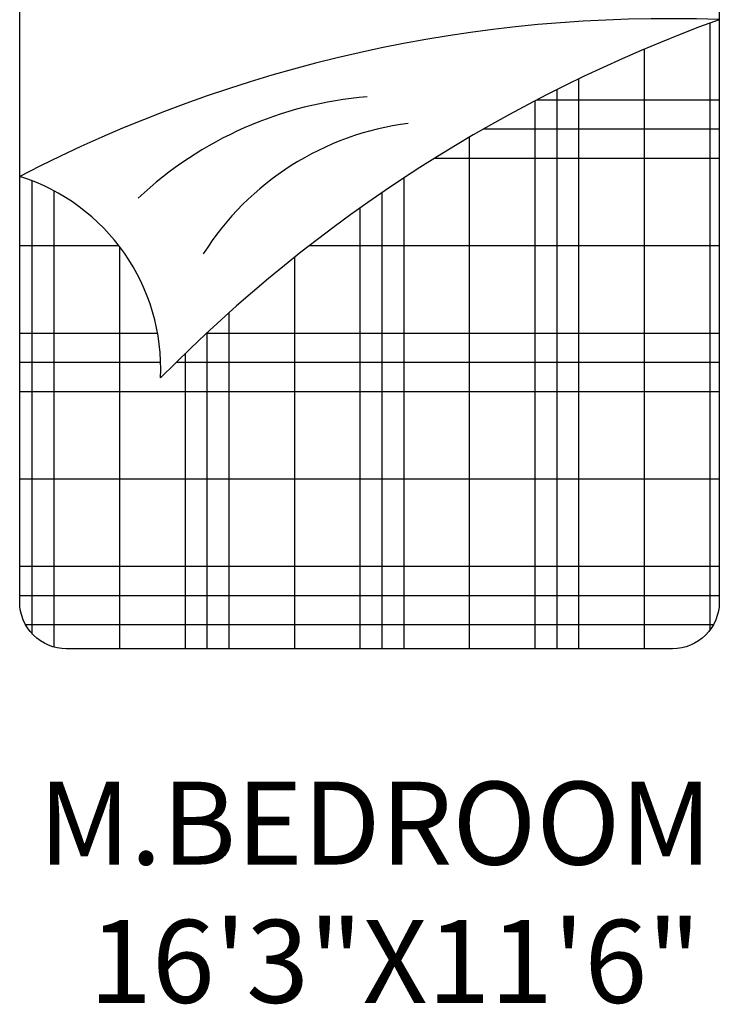
# Model space of a CAD drawing. Units: inches. Extents: x 3064 to 19385, y 846 to 15425.
# Tile 104 of 108: x 7735 to 7794, y 1289 to 1373. Entities that reach past the tile are written whole.
import ezdxf

# ---------------------------------------------------------------- set-up
doc = ezdxf.new("R2010")
doc.units = ezdxf.units.IN
doc.layers.add('A-AREA-IDEN', color=3, linetype='Continuous', lineweight=18)
doc.layers.add('A-FLOR-FIXT', color=9, linetype='Continuous', lineweight=18)
doc.layers.add('BLOCK', color=6, linetype='Continuous')
doc.styles.get("Standard").update_dxf_attribs({"font": 'arial.ttf'})

# ---------------------------------------------------------------- blocks, each defined once
blk = doc.blocks.new('*X5')
at = {"color": 0}
for p, q in [((276.598, 451.25), (280.51, 451.25)), ((275.455, 450.625), (280.51, 450.625)), ((274.411, 450), (280.51, 450)), ((265.51, 448.125), (267.634, 448.125)), ((271.723, 448.125), (280.51, 448.125)), ((265.51, 446.25), (268.465, 446.25)), ((269.519, 446.25), (280.51, 446.25)), ((265.51, 445.625), (268.531, 445.625)), ((268.866, 445.625), (280.51, 445.625)), ((265.51, 445), (280.51, 445)), ((265.51, 443.125), (280.51, 443.125)), ((265.51, 441.25), (280.51, 441.25)), ((265.51, 440.625), (280.51, 440.625)), ((265.634, 440), (280.386, 440))]:
    blk.add_line(p, q, dxfattribs=at)
blk = doc.blocks.new('*X6')
at = {"color": 0}
for p, q in [((280.312, 439.886), (280.312, 452.896)), ((278.906, 439.482), (278.906, 452.338)), ((277.5, 439.482), (277.5, 451.702)), ((277.031, 439.482), (277.031, 451.471)), ((276.562, 439.482), (276.562, 451.231)), ((275.156, 439.482), (275.156, 450.451)), ((265.781, 439.797), (265.781, 449.511)), ((273.75, 439.482), (273.75, 449.576)), ((266.25, 439.517), (266.25, 449.296)), ((273.281, 439.482), (273.281, 449.261)), ((272.812, 439.482), (272.812, 448.934)), ((267.656, 439.482), (267.656, 448.095)), ((271.406, 439.482), (271.406, 447.876)), ((270, 439.482), (270, 446.689)), ((269.531, 439.482), (269.531, 446.262)), ((269.062, 439.482), (269.062, 445.817))]:
    blk.add_line(p, q, dxfattribs=at)
blk = doc.blocks.new('A$C52E67D0D')
at = {"layer": 'BLOCK'}
blk.add_lwpolyline([(1901, 0), (601, 0, -0.414214), (501, 100), (501, 1700, -0.414214), (601, 1800), (1901, 1800, -0.414214), (2001, 1700), (2001, 100, -0.414214)], format="xyb", close=True, dxfattribs=at)
for centre, radius, start, end in [((1888.6, -1664.5), 3015.3, 87.8642, 117.4001), ((3101, -1685.8), 3227.7, 109.926, 135.3977), ((1308.8, 377.9), 807.6, 94.4436, 133.2788), ((1410.8, 520.2), 610.8, 97.2157, 147.6656), ((371.4, 600.4), 432, 357.3792, 72.5379)]:
    blk.add_arc(centre, radius, start, end, dxfattribs=at)
at = {"layer": 'BLOCK', "xscale": 100, "yscale": 100, "zscale": 100}
for name in ['*X6', '*X5']:
    blk.add_blockref(name, (-26050, -43948.2), dxfattribs=at)

msp = doc.modelspace()

# ---------------------------------------------------------------- block references
at = {"layer": 'A-FLOR-FIXT', "xscale": 0.039370099999992, "yscale": 0.039370099999992, "zscale": 0.039370099999992}
msp.add_blockref('A$C52E67D0D', (7715.494, 1319.474), dxfattribs=at)

# ---------------------------------------------------------------- texts
at = {"layer": 'A-AREA-IDEN', "insert": (7736.803, 1308.253), "char_height": 7, "attachment_point": 1}
msp.add_mtext_dynamic_manual_height_columns('M.BEDROOM\\P  16\'3"X11\'6"', width=67.59241, gutter_width=12.5, heights=[0], dxfattribs=at)

doc.saveas('drawing.dxf')
